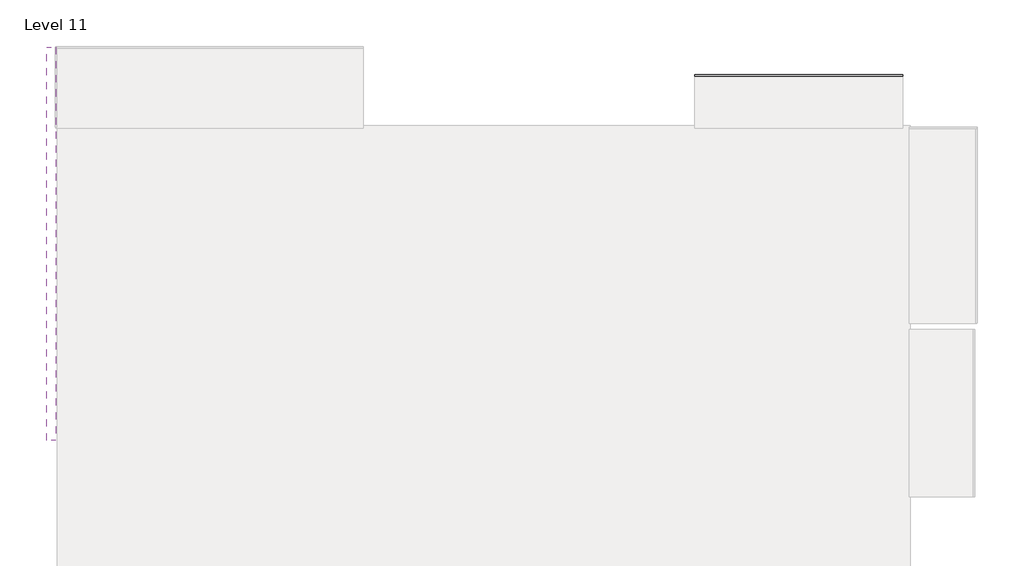
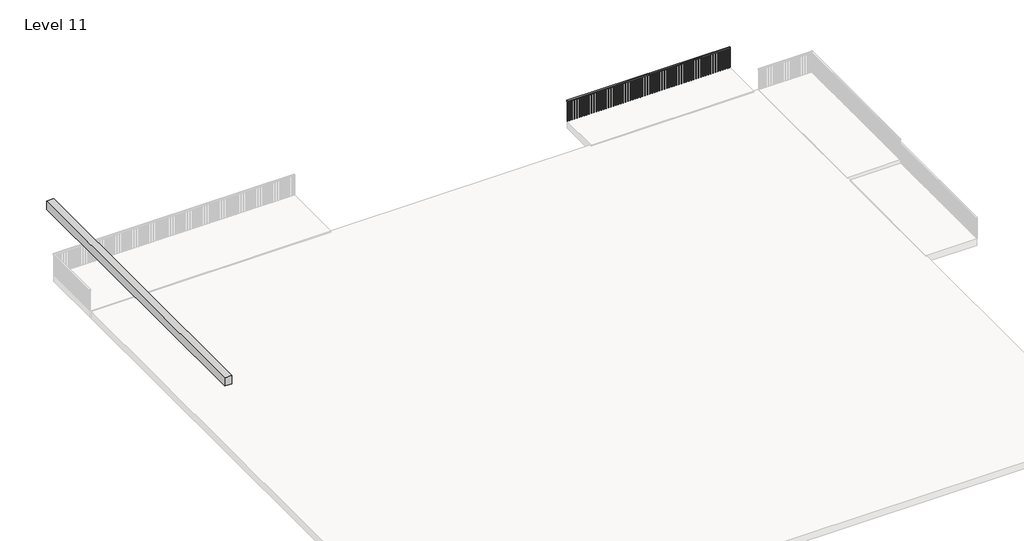
# One storey, part 5 of 5: 1 proxy, 1 railing.
"""IFC4 building model written with IfcOpenShell, lengths in millimetres."""

from ifc_helpers import new_model, si_unit, frame, origin, place, context, project, spatial, polyline, outline, extrude, transform, mapped, element, save
from components import generic_models_8_generic_models_8_16792cbe

model = new_model("IFC4")

# Units and contexts
model_context = context("Model", 3, world=origin())
ifc_project = project(units=[si_unit("LENGTHUNIT", "METRE", prefix="MILLI")], contexts=[model_context])

# Site, building, storey
site = spatial("IfcSite", under=ifc_project)
building = spatial("IfcBuilding", under=site)
storey = spatial("IfcBuildingStorey", under=building, Name="Level 11", Elevation=15544.8)

# Proxy
placement = place(None, origin())
generic_models_8_generic_models_8_shape = generic_models_8_generic_models_8_16792cbe(model_context)
element("IfcBuildingElementProxy", 1, Name="Generic Models 8 : Generic Models 8", ObjectType="Generic Models 8 : Generic Models 8", at=placement, inside=storey, context=model_context, shape_type="MappedRepresentation", body=[
    mapped(generic_models_8_generic_models_8_shape, transform((0.0, 0.0, 0.0), x_axis=(1.0, 0.0, 0.0), y_axis=(0.0, 1.0, 0.0), z_axis=(0.0, 0.0, 1.0))),
])

# Railing
element("IfcRailing", 2, ObjectType="Handrail - Rectangular", at=placement, inside=storey, context=model_context, shape_type="SweptSolid", body=[
    extrude(outline(polyline([(7096.1361222, 16470.4237525), (7096.1361222, 16521.2237525), (13903.3361222, 16521.2237525), (13903.3361222, 16470.4237525), (7096.1361222, 16470.4237525)])), frame((0.0, 0.0, 16408.4), z_axis=(0.0, 0.0, 1.0), x_axis=(1.0, 0.0, 0.0)), (0.0, 0.0, 1.0), 50.8),
    extrude(outline(polyline([(13792.2111222, 16486.2987525), (13792.2111222, 16505.3487525), (13811.2611222, 16505.3487525), (13811.2611222, 16486.2987525), (13792.2111222, 16486.2987525)])), frame((0.0, 0.0, 15544.8), z_axis=(0.0, 0.0, 1.0), x_axis=(1.0, 0.0, 0.0)), (0.0, 0.0, 1.0), 863.6),
    extrude(outline(polyline([(13690.6111222, 16486.2987525), (13690.6111222, 16505.3487525), (13709.6611222, 16505.3487525), (13709.6611222, 16486.2987525), (13690.6111222, 16486.2987525)])), frame((0.0, 0.0, 15544.8), z_axis=(0.0, 0.0, 1.0), x_axis=(1.0, 0.0, 0.0)), (0.0, 0.0, 1.0), 863.6),
    extrude(outline(polyline([(13589.0111222, 16486.2987525), (13589.0111222, 16505.3487525), (13608.0611222, 16505.3487525), (13608.0611222, 16486.2987525), (13589.0111222, 16486.2987525)])), frame((0.0, 0.0, 15544.8), z_axis=(0.0, 0.0, 1.0), x_axis=(1.0, 0.0, 0.0)), (0.0, 0.0, 1.0), 863.6),
    extrude(outline(polyline([(13487.4111222, 16486.2987525), (13487.4111222, 16505.3487525), (13506.4611222, 16505.3487525), (13506.4611222, 16486.2987525), (13487.4111222, 16486.2987525)])), frame((0.0, 0.0, 15544.8), z_axis=(0.0, 0.0, 1.0), x_axis=(1.0, 0.0, 0.0)), (0.0, 0.0, 1.0), 863.6),
    extrude(outline(polyline([(13385.8111222, 16486.2987525), (13385.8111222, 16505.3487525), (13404.8611222, 16505.3487525), (13404.8611222, 16486.2987525), (13385.8111222, 16486.2987525)])), frame((0.0, 0.0, 15544.8), z_axis=(0.0, 0.0, 1.0), x_axis=(1.0, 0.0, 0.0)), (0.0, 0.0, 1.0), 863.6),
    extrude(outline(polyline([(13284.2111222, 16486.2987525), (13284.2111222, 16505.3487525), (13303.2611222, 16505.3487525), (13303.2611222, 16486.2987525), (13284.2111222, 16486.2987525)])), frame((0.0, 0.0, 15544.8), z_axis=(0.0, 0.0, 1.0), x_axis=(1.0, 0.0, 0.0)), (0.0, 0.0, 1.0), 863.6),
    extrude(outline(polyline([(13182.6111222, 16486.2987525), (13182.6111222, 16505.3487525), (13201.6611222, 16505.3487525), (13201.6611222, 16486.2987525), (13182.6111222, 16486.2987525)])), frame((0.0, 0.0, 15544.8), z_axis=(0.0, 0.0, 1.0), x_axis=(1.0, 0.0, 0.0)), (0.0, 0.0, 1.0), 863.6),
    extrude(outline(polyline([(13081.0111222, 16486.2987525), (13081.0111222, 16505.3487525), (13100.0611222, 16505.3487525), (13100.0611222, 16486.2987525), (13081.0111222, 16486.2987525)])), frame((0.0, 0.0, 15544.8), z_axis=(0.0, 0.0, 1.0), x_axis=(1.0, 0.0, 0.0)), (0.0, 0.0, 1.0), 863.6),
    extrude(outline(polyline([(12979.4111222, 16486.2987525), (12979.4111222, 16505.3487525), (12998.4611222, 16505.3487525), (12998.4611222, 16486.2987525), (12979.4111222, 16486.2987525)])), frame((0.0, 0.0, 15544.8), z_axis=(0.0, 0.0, 1.0), x_axis=(1.0, 0.0, 0.0)), (0.0, 0.0, 1.0), 863.6),
    extrude(outline(polyline([(12877.8111222, 16486.2987525), (12877.8111222, 16505.3487525), (12896.8611222, 16505.3487525), (12896.8611222, 16486.2987525), (12877.8111222, 16486.2987525)])), frame((0.0, 0.0, 15544.8), z_axis=(0.0, 0.0, 1.0), x_axis=(1.0, 0.0, 0.0)), (0.0, 0.0, 1.0), 863.6),
    extrude(outline(polyline([(12776.2111222, 16486.2987525), (12776.2111222, 16505.3487525), (12795.2611222, 16505.3487525), (12795.2611222, 16486.2987525), (12776.2111222, 16486.2987525)])), frame((0.0, 0.0, 15544.8), z_axis=(0.0, 0.0, 1.0), x_axis=(1.0, 0.0, 0.0)), (0.0, 0.0, 1.0), 863.6),
    extrude(outline(polyline([(12674.6111222, 16486.2987525), (12674.6111222, 16505.3487525), (12693.6611222, 16505.3487525), (12693.6611222, 16486.2987525), (12674.6111222, 16486.2987525)])), frame((0.0, 0.0, 15544.8), z_axis=(0.0, 0.0, 1.0), x_axis=(1.0, 0.0, 0.0)), (0.0, 0.0, 1.0), 863.6),
    extrude(outline(polyline([(12573.0111222, 16486.2987525), (12573.0111222, 16505.3487525), (12592.0611222, 16505.3487525), (12592.0611222, 16486.2987525), (12573.0111222, 16486.2987525)])), frame((0.0, 0.0, 15544.8), z_axis=(0.0, 0.0, 1.0), x_axis=(1.0, 0.0, 0.0)), (0.0, 0.0, 1.0), 863.6),
    extrude(outline(polyline([(12471.4111222, 16486.2987525), (12471.4111222, 16505.3487525), (12490.4611222, 16505.3487525), (12490.4611222, 16486.2987525), (12471.4111222, 16486.2987525)])), frame((0.0, 0.0, 15544.8), z_axis=(0.0, 0.0, 1.0), x_axis=(1.0, 0.0, 0.0)), (0.0, 0.0, 1.0), 863.6),
    extrude(outline(polyline([(12369.8111222, 16486.2987525), (12369.8111222, 16505.3487525), (12388.8611222, 16505.3487525), (12388.8611222, 16486.2987525), (12369.8111222, 16486.2987525)])), frame((0.0, 0.0, 15544.8), z_axis=(0.0, 0.0, 1.0), x_axis=(1.0, 0.0, 0.0)), (0.0, 0.0, 1.0), 863.6),
    extrude(outline(polyline([(12268.2111222, 16486.2987525), (12268.2111222, 16505.3487525), (12287.2611222, 16505.3487525), (12287.2611222, 16486.2987525), (12268.2111222, 16486.2987525)])), frame((0.0, 0.0, 15544.8), z_axis=(0.0, 0.0, 1.0), x_axis=(1.0, 0.0, 0.0)), (0.0, 0.0, 1.0), 863.6),
    extrude(outline(polyline([(12166.6111222, 16486.2987525), (12166.6111222, 16505.3487525), (12185.6611222, 16505.3487525), (12185.6611222, 16486.2987525), (12166.6111222, 16486.2987525)])), frame((0.0, 0.0, 15544.8), z_axis=(0.0, 0.0, 1.0), x_axis=(1.0, 0.0, 0.0)), (0.0, 0.0, 1.0), 863.6),
    extrude(outline(polyline([(12065.0111222, 16486.2987525), (12065.0111222, 16505.3487525), (12084.0611222, 16505.3487525), (12084.0611222, 16486.2987525), (12065.0111222, 16486.2987525)])), frame((0.0, 0.0, 15544.8), z_axis=(0.0, 0.0, 1.0), x_axis=(1.0, 0.0, 0.0)), (0.0, 0.0, 1.0), 863.6),
    extrude(outline(polyline([(11963.4111222, 16486.2987525), (11963.4111222, 16505.3487525), (11982.4611222, 16505.3487525), (11982.4611222, 16486.2987525), (11963.4111222, 16486.2987525)])), frame((0.0, 0.0, 15544.8), z_axis=(0.0, 0.0, 1.0), x_axis=(1.0, 0.0, 0.0)), (0.0, 0.0, 1.0), 863.6),
    extrude(outline(polyline([(11861.8111222, 16486.2987525), (11861.8111222, 16505.3487525), (11880.8611222, 16505.3487525), (11880.8611222, 16486.2987525), (11861.8111222, 16486.2987525)])), frame((0.0, 0.0, 15544.8), z_axis=(0.0, 0.0, 1.0), x_axis=(1.0, 0.0, 0.0)), (0.0, 0.0, 1.0), 863.6),
    extrude(outline(polyline([(11760.2111222, 16486.2987525), (11760.2111222, 16505.3487525), (11779.2611222, 16505.3487525), (11779.2611222, 16486.2987525), (11760.2111222, 16486.2987525)])), frame((0.0, 0.0, 15544.8), z_axis=(0.0, 0.0, 1.0), x_axis=(1.0, 0.0, 0.0)), (0.0, 0.0, 1.0), 863.6),
    extrude(outline(polyline([(11658.6111222, 16486.2987525), (11658.6111222, 16505.3487525), (11677.6611222, 16505.3487525), (11677.6611222, 16486.2987525), (11658.6111222, 16486.2987525)])), frame((0.0, 0.0, 15544.8), z_axis=(0.0, 0.0, 1.0), x_axis=(1.0, 0.0, 0.0)), (0.0, 0.0, 1.0), 863.6),
    extrude(outline(polyline([(11557.0111222, 16486.2987525), (11557.0111222, 16505.3487525), (11576.0611222, 16505.3487525), (11576.0611222, 16486.2987525), (11557.0111222, 16486.2987525)])), frame((0.0, 0.0, 15544.8), z_axis=(0.0, 0.0, 1.0), x_axis=(1.0, 0.0, 0.0)), (0.0, 0.0, 1.0), 863.6),
    extrude(outline(polyline([(11455.4111222, 16486.2987525), (11455.4111222, 16505.3487525), (11474.4611222, 16505.3487525), (11474.4611222, 16486.2987525), (11455.4111222, 16486.2987525)])), frame((0.0, 0.0, 15544.8), z_axis=(0.0, 0.0, 1.0), x_axis=(1.0, 0.0, 0.0)), (0.0, 0.0, 1.0), 863.6),
    extrude(outline(polyline([(11353.8111222, 16486.2987525), (11353.8111222, 16505.3487525), (11372.8611222, 16505.3487525), (11372.8611222, 16486.2987525), (11353.8111222, 16486.2987525)])), frame((0.0, 0.0, 15544.8), z_axis=(0.0, 0.0, 1.0), x_axis=(1.0, 0.0, 0.0)), (0.0, 0.0, 1.0), 863.6),
    extrude(outline(polyline([(11252.2111222, 16486.2987525), (11252.2111222, 16505.3487525), (11271.2611222, 16505.3487525), (11271.2611222, 16486.2987525), (11252.2111222, 16486.2987525)])), frame((0.0, 0.0, 15544.8), z_axis=(0.0, 0.0, 1.0), x_axis=(1.0, 0.0, 0.0)), (0.0, 0.0, 1.0), 863.6),
    extrude(outline(polyline([(11150.6111222, 16486.2987525), (11150.6111222, 16505.3487525), (11169.6611222, 16505.3487525), (11169.6611222, 16486.2987525), (11150.6111222, 16486.2987525)])), frame((0.0, 0.0, 15544.8), z_axis=(0.0, 0.0, 1.0), x_axis=(1.0, 0.0, 0.0)), (0.0, 0.0, 1.0), 863.6),
    extrude(outline(polyline([(11049.0111222, 16486.2987525), (11049.0111222, 16505.3487525), (11068.0611222, 16505.3487525), (11068.0611222, 16486.2987525), (11049.0111222, 16486.2987525)])), frame((0.0, 0.0, 15544.8), z_axis=(0.0, 0.0, 1.0), x_axis=(1.0, 0.0, 0.0)), (0.0, 0.0, 1.0), 863.6),
    extrude(outline(polyline([(10947.4111222, 16486.2987525), (10947.4111222, 16505.3487525), (10966.4611222, 16505.3487525), (10966.4611222, 16486.2987525), (10947.4111222, 16486.2987525)])), frame((0.0, 0.0, 15544.8), z_axis=(0.0, 0.0, 1.0), x_axis=(1.0, 0.0, 0.0)), (0.0, 0.0, 1.0), 863.6),
    extrude(outline(polyline([(10845.8111222, 16486.2987525), (10845.8111222, 16505.3487525), (10864.8611222, 16505.3487525), (10864.8611222, 16486.2987525), (10845.8111222, 16486.2987525)])), frame((0.0, 0.0, 15544.8), z_axis=(0.0, 0.0, 1.0), x_axis=(1.0, 0.0, 0.0)), (0.0, 0.0, 1.0), 863.6),
    extrude(outline(polyline([(10744.2111222, 16486.2987525), (10744.2111222, 16505.3487525), (10763.2611222, 16505.3487525), (10763.2611222, 16486.2987525), (10744.2111222, 16486.2987525)])), frame((0.0, 0.0, 15544.8), z_axis=(0.0, 0.0, 1.0), x_axis=(1.0, 0.0, 0.0)), (0.0, 0.0, 1.0), 863.6),
    extrude(outline(polyline([(10642.6111222, 16486.2987525), (10642.6111222, 16505.3487525), (10661.6611222, 16505.3487525), (10661.6611222, 16486.2987525), (10642.6111222, 16486.2987525)])), frame((0.0, 0.0, 15544.8), z_axis=(0.0, 0.0, 1.0), x_axis=(1.0, 0.0, 0.0)), (0.0, 0.0, 1.0), 863.6),
    extrude(outline(polyline([(10541.0111222, 16486.2987525), (10541.0111222, 16505.3487525), (10560.0611222, 16505.3487525), (10560.0611222, 16486.2987525), (10541.0111222, 16486.2987525)])), frame((0.0, 0.0, 15544.8), z_axis=(0.0, 0.0, 1.0), x_axis=(1.0, 0.0, 0.0)), (0.0, 0.0, 1.0), 863.6),
    extrude(outline(polyline([(10439.4111222, 16486.2987525), (10439.4111222, 16505.3487525), (10458.4611222, 16505.3487525), (10458.4611222, 16486.2987525), (10439.4111222, 16486.2987525)])), frame((0.0, 0.0, 15544.8), z_axis=(0.0, 0.0, 1.0), x_axis=(1.0, 0.0, 0.0)), (0.0, 0.0, 1.0), 863.6),
    extrude(outline(polyline([(10337.8111222, 16486.2987525), (10337.8111222, 16505.3487525), (10356.8611222, 16505.3487525), (10356.8611222, 16486.2987525), (10337.8111222, 16486.2987525)])), frame((0.0, 0.0, 15544.8), z_axis=(0.0, 0.0, 1.0), x_axis=(1.0, 0.0, 0.0)), (0.0, 0.0, 1.0), 863.6),
    extrude(outline(polyline([(10236.2111222, 16486.2987525), (10236.2111222, 16505.3487525), (10255.2611222, 16505.3487525), (10255.2611222, 16486.2987525), (10236.2111222, 16486.2987525)])), frame((0.0, 0.0, 15544.8), z_axis=(0.0, 0.0, 1.0), x_axis=(1.0, 0.0, 0.0)), (0.0, 0.0, 1.0), 863.6),
    extrude(outline(polyline([(10134.6111222, 16486.2987525), (10134.6111222, 16505.3487525), (10153.6611222, 16505.3487525), (10153.6611222, 16486.2987525), (10134.6111222, 16486.2987525)])), frame((0.0, 0.0, 15544.8), z_axis=(0.0, 0.0, 1.0), x_axis=(1.0, 0.0, 0.0)), (0.0, 0.0, 1.0), 863.6),
    extrude(outline(polyline([(10033.0111222, 16486.2987525), (10033.0111222, 16505.3487525), (10052.0611222, 16505.3487525), (10052.0611222, 16486.2987525), (10033.0111222, 16486.2987525)])), frame((0.0, 0.0, 15544.8), z_axis=(0.0, 0.0, 1.0), x_axis=(1.0, 0.0, 0.0)), (0.0, 0.0, 1.0), 863.6),
    extrude(outline(polyline([(9931.4111222, 16486.2987525), (9931.4111222, 16505.3487525), (9950.4611222, 16505.3487525), (9950.4611222, 16486.2987525), (9931.4111222, 16486.2987525)])), frame((0.0, 0.0, 15544.8), z_axis=(0.0, 0.0, 1.0), x_axis=(1.0, 0.0, 0.0)), (0.0, 0.0, 1.0), 863.6),
    extrude(outline(polyline([(9829.8111222, 16486.2987525), (9829.8111222, 16505.3487525), (9848.8611222, 16505.3487525), (9848.8611222, 16486.2987525), (9829.8111222, 16486.2987525)])), frame((0.0, 0.0, 15544.8), z_axis=(0.0, 0.0, 1.0), x_axis=(1.0, 0.0, 0.0)), (0.0, 0.0, 1.0), 863.6),
    extrude(outline(polyline([(9728.2111222, 16486.2987525), (9728.2111222, 16505.3487525), (9747.2611222, 16505.3487525), (9747.2611222, 16486.2987525), (9728.2111222, 16486.2987525)])), frame((0.0, 0.0, 15544.8), z_axis=(0.0, 0.0, 1.0), x_axis=(1.0, 0.0, 0.0)), (0.0, 0.0, 1.0), 863.6),
    extrude(outline(polyline([(9626.6111222, 16486.2987525), (9626.6111222, 16505.3487525), (9645.6611222, 16505.3487525), (9645.6611222, 16486.2987525), (9626.6111222, 16486.2987525)])), frame((0.0, 0.0, 15544.8), z_axis=(0.0, 0.0, 1.0), x_axis=(1.0, 0.0, 0.0)), (0.0, 0.0, 1.0), 863.6),
    extrude(outline(polyline([(9525.0111222, 16486.2987525), (9525.0111222, 16505.3487525), (9544.0611222, 16505.3487525), (9544.0611222, 16486.2987525), (9525.0111222, 16486.2987525)])), frame((0.0, 0.0, 15544.8), z_axis=(0.0, 0.0, 1.0), x_axis=(1.0, 0.0, 0.0)), (0.0, 0.0, 1.0), 863.6),
    extrude(outline(polyline([(9423.4111222, 16486.2987525), (9423.4111222, 16505.3487525), (9442.4611222, 16505.3487525), (9442.4611222, 16486.2987525), (9423.4111222, 16486.2987525)])), frame((0.0, 0.0, 15544.8), z_axis=(0.0, 0.0, 1.0), x_axis=(1.0, 0.0, 0.0)), (0.0, 0.0, 1.0), 863.6),
    extrude(outline(polyline([(9321.8111222, 16486.2987525), (9321.8111222, 16505.3487525), (9340.8611222, 16505.3487525), (9340.8611222, 16486.2987525), (9321.8111222, 16486.2987525)])), frame((0.0, 0.0, 15544.8), z_axis=(0.0, 0.0, 1.0), x_axis=(1.0, 0.0, 0.0)), (0.0, 0.0, 1.0), 863.6),
    extrude(outline(polyline([(9220.2111222, 16486.2987525), (9220.2111222, 16505.3487525), (9239.2611222, 16505.3487525), (9239.2611222, 16486.2987525), (9220.2111222, 16486.2987525)])), frame((0.0, 0.0, 15544.8), z_axis=(0.0, 0.0, 1.0), x_axis=(1.0, 0.0, 0.0)), (0.0, 0.0, 1.0), 863.6),
    extrude(outline(polyline([(9118.6111222, 16486.2987525), (9118.6111222, 16505.3487525), (9137.6611222, 16505.3487525), (9137.6611222, 16486.2987525), (9118.6111222, 16486.2987525)])), frame((0.0, 0.0, 15544.8), z_axis=(0.0, 0.0, 1.0), x_axis=(1.0, 0.0, 0.0)), (0.0, 0.0, 1.0), 863.6),
    extrude(outline(polyline([(9017.0111222, 16486.2987525), (9017.0111222, 16505.3487525), (9036.0611222, 16505.3487525), (9036.0611222, 16486.2987525), (9017.0111222, 16486.2987525)])), frame((0.0, 0.0, 15544.8), z_axis=(0.0, 0.0, 1.0), x_axis=(1.0, 0.0, 0.0)), (0.0, 0.0, 1.0), 863.6),
    extrude(outline(polyline([(8915.4111222, 16486.2987525), (8915.4111222, 16505.3487525), (8934.4611222, 16505.3487525), (8934.4611222, 16486.2987525), (8915.4111222, 16486.2987525)])), frame((0.0, 0.0, 15544.8), z_axis=(0.0, 0.0, 1.0), x_axis=(1.0, 0.0, 0.0)), (0.0, 0.0, 1.0), 863.6),
    extrude(outline(polyline([(8813.8111222, 16486.2987525), (8813.8111222, 16505.3487525), (8832.8611222, 16505.3487525), (8832.8611222, 16486.2987525), (8813.8111222, 16486.2987525)])), frame((0.0, 0.0, 15544.8), z_axis=(0.0, 0.0, 1.0), x_axis=(1.0, 0.0, 0.0)), (0.0, 0.0, 1.0), 863.6),
    extrude(outline(polyline([(8712.2111222, 16486.2987525), (8712.2111222, 16505.3487525), (8731.2611222, 16505.3487525), (8731.2611222, 16486.2987525), (8712.2111222, 16486.2987525)])), frame((0.0, 0.0, 15544.8), z_axis=(0.0, 0.0, 1.0), x_axis=(1.0, 0.0, 0.0)), (0.0, 0.0, 1.0), 863.6),
    extrude(outline(polyline([(8610.6111222, 16486.2987525), (8610.6111222, 16505.3487525), (8629.6611222, 16505.3487525), (8629.6611222, 16486.2987525), (8610.6111222, 16486.2987525)])), frame((0.0, 0.0, 15544.8), z_axis=(0.0, 0.0, 1.0), x_axis=(1.0, 0.0, 0.0)), (0.0, 0.0, 1.0), 863.6),
    extrude(outline(polyline([(8509.0111222, 16486.2987525), (8509.0111222, 16505.3487525), (8528.0611222, 16505.3487525), (8528.0611222, 16486.2987525), (8509.0111222, 16486.2987525)])), frame((0.0, 0.0, 15544.8), z_axis=(0.0, 0.0, 1.0), x_axis=(1.0, 0.0, 0.0)), (0.0, 0.0, 1.0), 863.6),
    extrude(outline(polyline([(8407.4111222, 16486.2987525), (8407.4111222, 16505.3487525), (8426.4611222, 16505.3487525), (8426.4611222, 16486.2987525), (8407.4111222, 16486.2987525)])), frame((0.0, 0.0, 15544.8), z_axis=(0.0, 0.0, 1.0), x_axis=(1.0, 0.0, 0.0)), (0.0, 0.0, 1.0), 863.6),
    extrude(outline(polyline([(8305.8111222, 16486.2987525), (8305.8111222, 16505.3487525), (8324.8611222, 16505.3487525), (8324.8611222, 16486.2987525), (8305.8111222, 16486.2987525)])), frame((0.0, 0.0, 15544.8), z_axis=(0.0, 0.0, 1.0), x_axis=(1.0, 0.0, 0.0)), (0.0, 0.0, 1.0), 863.6),
    extrude(outline(polyline([(8204.2111222, 16486.2987525), (8204.2111222, 16505.3487525), (8223.2611222, 16505.3487525), (8223.2611222, 16486.2987525), (8204.2111222, 16486.2987525)])), frame((0.0, 0.0, 15544.8), z_axis=(0.0, 0.0, 1.0), x_axis=(1.0, 0.0, 0.0)), (0.0, 0.0, 1.0), 863.6),
    extrude(outline(polyline([(8102.6111222, 16486.2987525), (8102.6111222, 16505.3487525), (8121.6611222, 16505.3487525), (8121.6611222, 16486.2987525), (8102.6111222, 16486.2987525)])), frame((0.0, 0.0, 15544.8), z_axis=(0.0, 0.0, 1.0), x_axis=(1.0, 0.0, 0.0)), (0.0, 0.0, 1.0), 863.6),
    extrude(outline(polyline([(8001.0111222, 16486.2987525), (8001.0111222, 16505.3487525), (8020.0611222, 16505.3487525), (8020.0611222, 16486.2987525), (8001.0111222, 16486.2987525)])), frame((0.0, 0.0, 15544.8), z_axis=(0.0, 0.0, 1.0), x_axis=(1.0, 0.0, 0.0)), (0.0, 0.0, 1.0), 863.6),
    extrude(outline(polyline([(7899.4111222, 16486.2987525), (7899.4111222, 16505.3487525), (7918.4611222, 16505.3487525), (7918.4611222, 16486.2987525), (7899.4111222, 16486.2987525)])), frame((0.0, 0.0, 15544.8), z_axis=(0.0, 0.0, 1.0), x_axis=(1.0, 0.0, 0.0)), (0.0, 0.0, 1.0), 863.6),
    extrude(outline(polyline([(7797.8111222, 16486.2987525), (7797.8111222, 16505.3487525), (7816.8611222, 16505.3487525), (7816.8611222, 16486.2987525), (7797.8111222, 16486.2987525)])), frame((0.0, 0.0, 15544.8), z_axis=(0.0, 0.0, 1.0), x_axis=(1.0, 0.0, 0.0)), (0.0, 0.0, 1.0), 863.6),
    extrude(outline(polyline([(7696.2111222, 16486.2987525), (7696.2111222, 16505.3487525), (7715.2611222, 16505.3487525), (7715.2611222, 16486.2987525), (7696.2111222, 16486.2987525)])), frame((0.0, 0.0, 15544.8), z_axis=(0.0, 0.0, 1.0), x_axis=(1.0, 0.0, 0.0)), (0.0, 0.0, 1.0), 863.6),
    extrude(outline(polyline([(7594.6111222, 16486.2987525), (7594.6111222, 16505.3487525), (7613.6611222, 16505.3487525), (7613.6611222, 16486.2987525), (7594.6111222, 16486.2987525)])), frame((0.0, 0.0, 15544.8), z_axis=(0.0, 0.0, 1.0), x_axis=(1.0, 0.0, 0.0)), (0.0, 0.0, 1.0), 863.6),
    extrude(outline(polyline([(7493.0111222, 16486.2987525), (7493.0111222, 16505.3487525), (7512.0611222, 16505.3487525), (7512.0611222, 16486.2987525), (7493.0111222, 16486.2987525)])), frame((0.0, 0.0, 15544.8), z_axis=(0.0, 0.0, 1.0), x_axis=(1.0, 0.0, 0.0)), (0.0, 0.0, 1.0), 863.6),
    extrude(outline(polyline([(7391.4111222, 16486.2987525), (7391.4111222, 16505.3487525), (7410.4611222, 16505.3487525), (7410.4611222, 16486.2987525), (7391.4111222, 16486.2987525)])), frame((0.0, 0.0, 15544.8), z_axis=(0.0, 0.0, 1.0), x_axis=(1.0, 0.0, 0.0)), (0.0, 0.0, 1.0), 863.6),
    extrude(outline(polyline([(7289.8111222, 16486.2987525), (7289.8111222, 16505.3487525), (7308.8611222, 16505.3487525), (7308.8611222, 16486.2987525), (7289.8111222, 16486.2987525)])), frame((0.0, 0.0, 15544.8), z_axis=(0.0, 0.0, 1.0), x_axis=(1.0, 0.0, 0.0)), (0.0, 0.0, 1.0), 863.6),
    extrude(outline(polyline([(7188.2111222, 16486.2987525), (7188.2111222, 16505.3487525), (7207.2611222, 16505.3487525), (7207.2611222, 16486.2987525), (7188.2111222, 16486.2987525)])), frame((0.0, 0.0, 15544.8), z_axis=(0.0, 0.0, 1.0), x_axis=(1.0, 0.0, 0.0)), (0.0, 0.0, 1.0), 863.6),
    extrude(outline(polyline([(13884.2861222, 16486.2987525), (13884.2861222, 16505.3487525), (13903.3361222, 16505.3487525), (13903.3361222, 16486.2987525), (13884.2861222, 16486.2987525)])), frame((0.0, 0.0, 15544.8), z_axis=(0.0, 0.0, 1.0), x_axis=(1.0, 0.0, 0.0)), (0.0, 0.0, 1.0), 863.6),
    extrude(outline(polyline([(7096.1361222, 16486.2987525), (7096.1361222, 16505.3487525), (7115.1861222, 16505.3487525), (7115.1861222, 16486.2987525), (7096.1361222, 16486.2987525)])), frame((0.0, 0.0, 15544.8), z_axis=(0.0, 0.0, 1.0), x_axis=(1.0, 0.0, 0.0)), (0.0, 0.0, 1.0), 863.6),
])

save(model, "model.ifc")

# Revit data of these elements
# Type "Handrail - Rectangular"
#   Assembly Code = "C2010400"
#   built-in parameter 1008612 = 0.0416667 (stored number, unit not read)
#   built-in parameter 1008611 = 0.0416667 (stored number, unit not read)
#   built-in parameter 1008609 = 0.333333 (stored number, unit not read)
#   built-in parameter 1008604 = 0.166667 (stored number, unit not read)
#   built-in parameter 1008603 = 0.166667 (stored number, unit not read)
#   Railing Height = 3' - 0"
#   built-in parameter 1008630 = 2
#   built-in parameter 1008610 = 2
#   built-in parameter 1008618 = Baluster - Square : 3/4"
# Element 1 (IfcBuildingElementProxy, "Generic Models 8 : Generic Models 8")
#   Phase Created = New Construction
# Element 2 (IfcRailing, "Handrail - Rectangular")
#   Phase Created = New Construction
